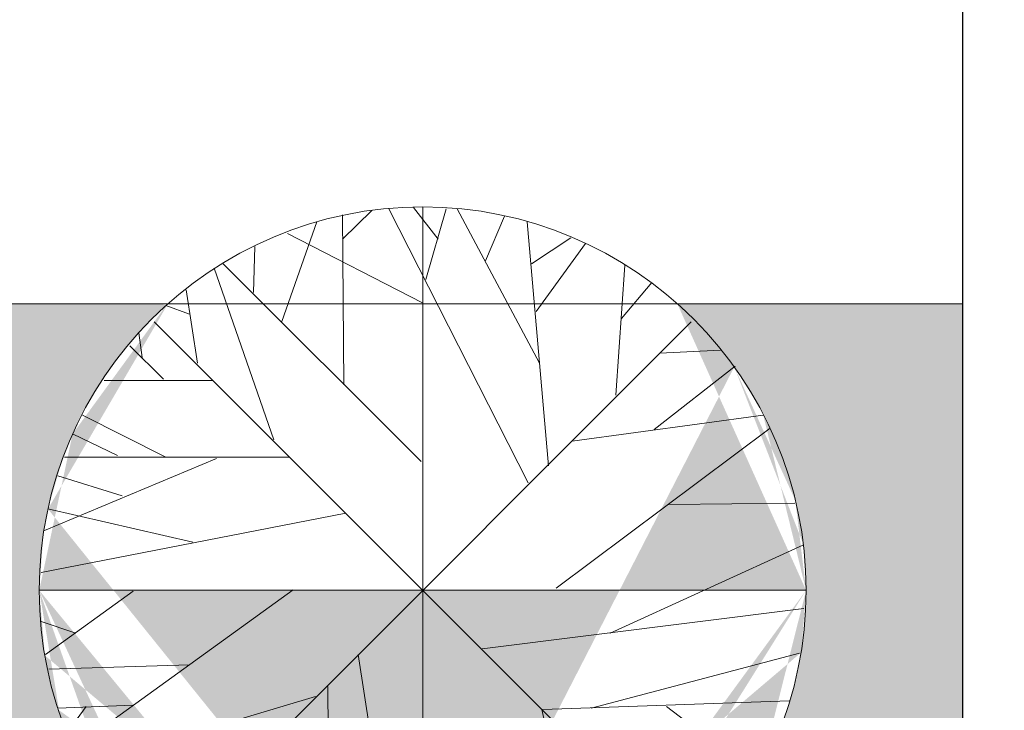
# Model space of a CAD drawing. Units: inches. Extents: x 459864 to 460310, y 324185 to 324787.
# Tile 77 of 112: x 460240 to 460271, y 324260 to 324281. Entities that reach past the tile are written whole.
import ezdxf

# ---------------------------------------------------------------- set-up
doc = ezdxf.new("R2010")
doc.units = ezdxf.units.IN
for name, color, linetype, lineweight in [('A-ANNO-DIMS', 2, 'Continuous', 18), ('C-PROP', 7, 'Continuous', 30), ('L-PLNT', 3, 'Continuous', 13), ('L-SITE-PATT', 252, 'Continuous', 13)]:
    doc.layers.add(name, color=color, linetype=linetype, lineweight=lineweight)
doc.styles.get("Standard").update_dxf_attribs({"font": 'arial.ttf'})
doc.dimstyles.new('ISO-25', dxfattribs={"dimtxt": 6, "dimasz": 2.5, "dimexe": 1.25, "dimexo": 0.625, "dimtad": 1, "dimdec": 1, "dimlunit": 3, "dimtxsty": 'Standard', "dimcen": 2.5, "dimadec": 0, "dimazin": 0, "dimtfac": 1, "dimtdec": 1, "dimtmove": 0, "dimatfit": 3, "dimfxl": 1, "dimarcsym": 0})

# ---------------------------------------------------------------- blocks, each defined once
blk = doc.blocks.new('Tree - deciduous plan')
for p, q in [((-12.5388, 54.9406), (-7.9613, 59.4546)), ((-12.3627, 32.1443), (-12.5388, 58.7776)), ((-5.3205, 59.6806), (16.5105, 16.7963)), ((2.426, 54.9406), (-1.4472, 59.9056)), ((0, 59.9996), (0, -60)), ((0.4894, 48.6208), (3.6584, 59.6806)), ((18.2711, 35.5298), (5.419, 59.6806)), ((9.8203, 51.5549), (12.8133, 58.5516)), ((-22.0458, 42.0753), (-16.5881, 57.6486)), ((19.6795, 19.5047), (16.3344, 57.6486)), ((-21.1656, 55.8436), (-0.0388, 45.0094)), ((17.0387, 51.1035), (23.2006, 55.1666)), ((17.7429, 43.6552), (25.4894, 54.2636)), ((-26.4472, 46.5894), (-26.2712, 53.8116)), ((-31.2008, 51.1035), (-0.2149, 20.1818)), ((31.6513, 50.8778), (30.2429, 30.5643)), ((-32.6092, 50.4264), (-23.2782, 23.5674)), ((31.1232, 42.5267), (35.8767, 48.1693)), ((-37.0107, 47.0408), (-35.25, 35.5298)), ((-40.1797, 44.558), (-36.4825, 43.2038)), ((42, 42), (-42, -42)), ((42, -42), (-42, 42)), ((-43.8768, 36.4326), (-44.405, 40.2696)), ((-45.8134, 38.2383), (-40.5318, 33.0471)), ((37.1091, 37.1098), (46.6161, 37.5612)), ((36.2288, 25.1474), (48.9049, 35.0784)), ((-49.8627, 32.8214), (-32.7853, 32.8214)), ((-53.2078, 27.4044), (-40.1797, 20.859)), ((23.3767, 23.3417), (53.3063, 27.4044)), ((54.3626, 25.3731), (20.9119, 0.3198)), ((-54.7923, 24.4702), (-47.75, 21.0847)), ((-32.2571, 20.6333), (-59.1937, 9.348)), ((-56.0247, 20.859), (-20.8134, 20.859)), ((-57.081, 17.9248), (-47.0458, 14.7649)), ((-58.6656, 12.7336), (-35.9543, 7.5424)), ((38.5175, 13.4107), (58.2359, 13.6364)), ((-59.7219, 2.8025), (-12.0106, 12.0565)), ((29.3626, -6.6771), (59.4682, 7.091)), ((-54.6162, -24.7335), (-20.2853, 0.0941)), ((-60, 0), (60, 0)), ((-45.2853, -0.1316), (-59.0177, -10.0627)), ((9.2922, -9.1598), (59.6443, -2.8401)), ((-59.7219, -4.8714), (-54.2641, -6.6771)), ((-10.074, -10.0627), (-2.5036, -59.7178)), ((26.3697, -18.4138), (58.9401, -9.8369)), ((-58.4895, -12.3197), (-36.4825, -11.6426)), ((-14.8275, -15.0282), (-14.6515, -57.6865)), ((-53.2078, -27.442), (-16.7641, -16.6081)), ((-57.081, -18.4138), (-45.2853, -17.9624)), ((-52.6797, -18.188), (-55.4966, -22.0251)), ((18.7992, -18.6394), (57.3556, -17.2853)), ((38.1654, -18.188), (52.426, -29.0219)), ((18.6232, -18.6394), (26.7218, -53.3981))]:
    blk.add_line(p, q)
blk.add_circle((0, 0), 60)
blk = doc.blocks.new('*D65')
at = {"layer": 'A-ANNO-DIMS', "color": 0, "lineweight": -2, "transparency": 16777216}
for p, q in [((460247.74, 324283.483), (460302.765, 324283.483)), ((460301.515, 324280.983), (460301.515, 324197.483)), ((460271.74, 324194.983), (460302.765, 324194.983))]:
    blk.add_line(p, q, dxfattribs=at)
at = {"layer": 'A-ANNO-DIMS', "color": 0, "transparency": 16777216}
for points in [[(460301.098, 324280.983), (460301.932, 324280.983), (460301.515, 324283.483)], [(460301.098, 324197.483), (460301.932, 324197.483), (460301.515, 324194.983)]]:
    blk.add_solid(points, dxfattribs=at)
at = {"layer": 'Defpoints', "color": 0, "transparency": 16777216}
for p in [(460247.115, 324283.483), (460271.115, 324194.983), (460301.515, 324194.983)]:
    blk.add_point(p, dxfattribs=at)
at = {"layer": 'A-ANNO-DIMS', "color": 0, "transparency": 16777216, "insert": (460297.788, 324239.233), "char_height": 6, "attachment_point": 5, "rotation": 90}
blk.add_mtext('7\'-4 1/2"', dxfattribs=at)

msp = doc.modelspace()

# ---------------------------------------------------------------- hatches: boundary and pattern name
at = {"layer": 'L-SITE-PATT'}
h = msp.add_hatch(dxfattribs=at)
h.set_pattern_fill('DOTS', color=256)
h.paths.add_polyline_path([(460269.804, 324283.483), (460247.115, 324283.483), (460121.929, 324283.483), (460121.929, 324252.473), (460117.429, 324252.473), (460110.124, 324252.473), (460110.124, 324243.287), (460080.83, 324243.287), (460080.83, 324252.473), (460061.115, 324252.473), (460061.115, 324251.882), (460077.909, 324251.882), (460077.909, 324199.483), (460080.83, 324199.483), (460080.83, 324207.553), (460110.124, 324207.553), (460110.124, 324199.483), (460110.813, 324199.483), (460262.115, 324199.483), (460269.804, 324199.483)], flags=17)
edge = h.paths.add_edge_path(flags=0)
edge.add_ellipse((460222.59, 324263.813), major_axis=(-8.485, 8.485), ratio=1, start_angle=405, end_angle=495, ccw=False)
edge.add_line((460214.821, 324254.66), (460214.832, 324254.666))
edge.add_ellipse((460222.59, 324263.813), major_axis=(-8.485, 8.485), ratio=1, start_angle=405, end_angle=495, ccw=False)
edge.add_line((460210.759, 324261.781), (460210.768, 324261.787))
edge.add_ellipse((460222.59, 324263.813), major_axis=(-8.485, 8.485), ratio=1, start_angle=405, end_angle=495, ccw=False)
edge.add_ellipse((460222.59, 324263.813), major_axis=(-8.485, 8.485), ratio=1, start_angle=392.754, end_angle=405, ccw=False)
edge.add_ellipse((460222.59, 324263.813), major_axis=(-8.485, 8.485), ratio=1, start_angle=380.9347, end_angle=392.754, ccw=False)
edge.add_line((460211.337, 324267.985), (460211.34, 324267.985))
edge.add_ellipse((460222.59, 324263.813), major_axis=(-8.485, 8.485), ratio=1, start_angle=380.9347, end_angle=392.754, ccw=False)
edge.add_ellipse((460222.59, 324263.813), major_axis=(-8.485, 8.485), ratio=1, start_angle=347.9015, end_angle=380.9347, ccw=False)
edge.add_ellipse((460222.59, 324263.813), major_axis=(-8.485, 8.485), ratio=1, start_angle=327.0619, end_angle=347.9015, ccw=False)
edge.add_ellipse((460222.59, 324263.813), major_axis=(-8.485, 8.485), ratio=1, start_angle=278.3246, end_angle=327.0619, ccw=False)
edge.add_line((460225.158, 324275.536), (460225.158, 324275.535))
edge.add_ellipse((460222.59, 324263.813), major_axis=(-8.485, 8.485), ratio=1, start_angle=278.3246, end_angle=327.0619, ccw=False)
edge.add_ellipse((460222.59, 324263.813), major_axis=(-8.485, 8.485), ratio=1, start_angle=260.6436, end_angle=278.3246, ccw=False)
edge.add_ellipse((460222.59, 324263.813), major_axis=(-8.485, 8.485), ratio=1, start_angle=225, end_angle=260.6436, ccw=False)
edge.add_line((460234.509, 324265.243), (460234.501, 324265.239))
edge.add_ellipse((460222.59, 324263.813), major_axis=(-8.485, 8.485), ratio=1, start_angle=225, end_angle=260.6436, ccw=False)
edge.add_ellipse((460222.59, 324263.813), major_axis=(-8.485, 8.485), ratio=1, start_angle=495, end_angle=585, ccw=False)
edge.add_line((460234.437, 324261.861), (460234.424, 324261.858))
edge.add_ellipse((460222.59, 324263.813), major_axis=(-8.485, 8.485), ratio=1, start_angle=495, end_angle=585, ccw=False)
edge.add_line((460227.95, 324253.067), (460227.946, 324253.083))
edge.add_ellipse((460222.59, 324263.813), major_axis=(-8.485, 8.485), ratio=1, start_angle=495, end_angle=585, ccw=False)
edge.add_line((460226.223, 324252.369), (460226.211, 324252.38))
edge.add_ellipse((460222.59, 324263.813), major_axis=(-8.485, 8.485), ratio=1, start_angle=495, end_angle=585, ccw=False)
h.paths.add_polyline_path([(460219.651, 324254.347), (460218.461, 324253.545), (460218.275, 324254.789), (460219.642, 324256.542), (460219.625, 324260.848), (460216.11, 324257.333), (460214.35, 324256.978), (460215.416, 324259.356), (460212.524, 324258.496), (460213.137, 324259.93), (460218.507, 324263.813), (460222.59, 324263.813), (460222.59, 324267.807), (460218.176, 324272.212), (460219.026, 324274.639), (460222.59, 324272.811), (460222.59, 324275.423), (460223.057, 324274.825), (460222.675, 324273.492), (460225.912, 324267.135), (460219.625, 324260.848)], flags=0)
edge = h.paths.add_edge_path(flags=0)
edge.add_ellipse((460194.576, 324264.046), major_axis=(-8.485, 8.485), ratio=1, start_angle=495, end_angle=585, ccw=False)
edge.add_line((460199.936, 324253.3), (460199.932, 324253.316))
edge.add_ellipse((460194.576, 324264.046), major_axis=(-8.485, 8.485), ratio=1, start_angle=495, end_angle=585, ccw=False)
edge.add_line((460198.208, 324252.603), (460198.196, 324252.613))
edge.add_ellipse((460194.576, 324264.046), major_axis=(-8.485, 8.485), ratio=1, start_angle=495, end_angle=585, ccw=False)
edge.add_ellipse((460194.576, 324264.046), major_axis=(-8.485, 8.485), ratio=1, start_angle=405, end_angle=495, ccw=False)
edge.add_line((460186.806, 324254.893), (460186.817, 324254.899))
edge.add_ellipse((460194.576, 324264.046), major_axis=(-8.485, 8.485), ratio=1, start_angle=405, end_angle=495, ccw=False)
edge.add_line((460182.744, 324262.014), (460182.753, 324262.02))
edge.add_ellipse((460194.576, 324264.046), major_axis=(-8.485, 8.485), ratio=1, start_angle=405, end_angle=495, ccw=False)
edge.add_ellipse((460194.576, 324264.046), major_axis=(-8.485, 8.485), ratio=1, start_angle=392.754, end_angle=405, ccw=False)
edge.add_ellipse((460194.576, 324264.046), major_axis=(-8.485, 8.485), ratio=1, start_angle=380.9347, end_angle=392.754, ccw=False)
edge.add_line((460183.323, 324268.218), (460183.326, 324268.218))
edge.add_ellipse((460194.576, 324264.046), major_axis=(-8.485, 8.485), ratio=1, start_angle=380.9347, end_angle=392.754, ccw=False)
edge.add_ellipse((460194.576, 324264.046), major_axis=(-8.485, 8.485), ratio=1, start_angle=347.9015, end_angle=380.9347, ccw=False)
edge.add_ellipse((460194.576, 324264.046), major_axis=(-8.485, 8.485), ratio=1, start_angle=327.0619, end_angle=347.9015, ccw=False)
edge.add_ellipse((460194.576, 324264.046), major_axis=(-8.485, 8.485), ratio=1, start_angle=278.3246, end_angle=327.0619, ccw=False)
edge.add_line((460197.144, 324275.769), (460197.143, 324275.768))
edge.add_ellipse((460194.576, 324264.046), major_axis=(-8.485, 8.485), ratio=1, start_angle=278.3246, end_angle=327.0619, ccw=False)
edge.add_ellipse((460194.576, 324264.046), major_axis=(-8.485, 8.485), ratio=1, start_angle=260.6436, end_angle=278.3246, ccw=False)
edge.add_ellipse((460194.576, 324264.046), major_axis=(-8.485, 8.485), ratio=1, start_angle=225, end_angle=260.6436, ccw=False)
edge.add_line((460206.494, 324265.476), (460206.487, 324265.473))
edge.add_ellipse((460194.576, 324264.046), major_axis=(-8.485, 8.485), ratio=1, start_angle=225, end_angle=260.6436, ccw=False)
edge.add_ellipse((460194.576, 324264.046), major_axis=(-8.485, 8.485), ratio=1, start_angle=495, end_angle=585, ccw=False)
edge.add_line((460206.422, 324262.094), (460206.409, 324262.091))
h.paths.add_polyline_path([(460191.61, 324261.081), (460191.637, 324254.58), (460190.447, 324253.778), (460190.261, 324255.023), (460191.628, 324256.775), (460191.61, 324261.081), (460188.096, 324257.566), (460186.335, 324257.211), (460187.402, 324259.589), (460184.509, 324258.729), (460185.123, 324260.163), (460190.493, 324264.046), (460194.576, 324264.046), (460194.576, 324268.04), (460190.161, 324272.446), (460191.011, 324274.872), (460194.576, 324273.044), (460194.576, 324275.657), (460195.043, 324275.058), (460194.661, 324273.725), (460197.897, 324267.368)], flags=0)
edge = h.paths.add_edge_path(flags=0)
edge.add_ellipse((460252.912, 324263.578), major_axis=(-8.485, 8.485), ratio=1, start_angle=405, end_angle=495, ccw=False)
edge.add_line((460241.081, 324261.545), (460241.089, 324261.551))
edge.add_ellipse((460252.912, 324263.578), major_axis=(-8.485, 8.485), ratio=1, start_angle=405, end_angle=495, ccw=False)
edge.add_ellipse((460252.912, 324263.578), major_axis=(-8.485, 8.485), ratio=1, start_angle=392.754, end_angle=405, ccw=False)
edge.add_ellipse((460252.912, 324263.578), major_axis=(-8.485, 8.485), ratio=1, start_angle=380.9347, end_angle=392.754, ccw=False)
edge.add_line((460241.659, 324267.749), (460241.662, 324267.749))
edge.add_ellipse((460252.912, 324263.578), major_axis=(-8.485, 8.485), ratio=1, start_angle=380.9347, end_angle=392.754, ccw=False)
edge.add_ellipse((460252.912, 324263.578), major_axis=(-8.485, 8.485), ratio=1, start_angle=347.9015, end_angle=380.9347, ccw=False)
edge.add_ellipse((460252.912, 324263.578), major_axis=(-8.485, 8.485), ratio=1, start_angle=327.0619, end_angle=347.9015, ccw=False)
edge.add_ellipse((460252.912, 324263.578), major_axis=(-8.485, 8.485), ratio=1, start_angle=278.3246, end_angle=327.0619, ccw=False)
edge.add_line((460255.48, 324275.3), (460255.479, 324275.299))
edge.add_ellipse((460252.912, 324263.578), major_axis=(-8.485, 8.485), ratio=1, start_angle=278.3246, end_angle=327.0619, ccw=False)
edge.add_ellipse((460252.912, 324263.578), major_axis=(-8.485, 8.485), ratio=1, start_angle=260.6436, end_angle=278.3246, ccw=False)
edge.add_ellipse((460252.912, 324263.578), major_axis=(-8.485, 8.485), ratio=1, start_angle=225, end_angle=260.6436, ccw=False)
edge.add_line((460264.83, 324265.007), (460264.823, 324265.004))
edge.add_ellipse((460252.912, 324263.578), major_axis=(-8.485, 8.485), ratio=1, start_angle=225, end_angle=260.6436, ccw=False)
edge.add_ellipse((460252.912, 324263.578), major_axis=(-8.485, 8.485), ratio=1, start_angle=495, end_angle=585, ccw=False)
edge.add_line((460264.758, 324261.626), (460264.745, 324261.622))
edge.add_ellipse((460252.912, 324263.578), major_axis=(-8.485, 8.485), ratio=1, start_angle=495, end_angle=585, ccw=False)
edge.add_line((460258.272, 324252.832), (460258.268, 324252.848))
edge.add_ellipse((460252.912, 324263.578), major_axis=(-8.485, 8.485), ratio=1, start_angle=495, end_angle=585, ccw=False)
edge.add_line((460256.545, 324252.134), (460256.533, 324252.144))
edge.add_ellipse((460252.912, 324263.578), major_axis=(-8.485, 8.485), ratio=1, start_angle=495, end_angle=585, ccw=False)
edge.add_ellipse((460252.912, 324263.578), major_axis=(-8.485, 8.485), ratio=1, start_angle=405, end_angle=495, ccw=False)
edge.add_line((460245.143, 324254.424), (460245.153, 324254.43))
h.paths.add_polyline_path([(460244.672, 324256.742), (460245.738, 324259.12), (460242.846, 324258.26), (460243.459, 324259.694), (460248.829, 324263.578), (460252.912, 324263.578), (460252.912, 324267.571), (460248.497, 324271.977), (460249.348, 324274.403), (460252.912, 324272.576), (460252.912, 324275.188), (460253.379, 324274.589), (460252.997, 324273.257), (460256.233, 324266.899), (460249.946, 324260.612), (460249.973, 324254.111), (460248.783, 324253.309), (460248.597, 324254.554), (460249.964, 324256.306), (460249.946, 324260.612), (460246.432, 324257.097)], flags=0)
edge = h.paths.add_edge_path(flags=0)
edge.add_ellipse((460167.439, 324262.833), major_axis=(-8.485, 8.485), ratio=1, start_angle=495, end_angle=585, ccw=False)
edge.add_line((460172.799, 324252.087), (460172.795, 324252.103))
edge.add_ellipse((460167.439, 324262.833), major_axis=(-8.485, 8.485), ratio=1, start_angle=495, end_angle=585, ccw=False)
edge.add_line((460171.071, 324251.389), (460171.059, 324251.399))
edge.add_ellipse((460167.439, 324262.833), major_axis=(-8.485, 8.485), ratio=1, start_angle=495, end_angle=585, ccw=False)
edge.add_ellipse((460167.439, 324262.833), major_axis=(-8.485, 8.485), ratio=1, start_angle=405, end_angle=495, ccw=False)
edge.add_line((460159.669, 324253.679), (460159.68, 324253.685))
edge.add_ellipse((460167.439, 324262.833), major_axis=(-8.485, 8.485), ratio=1, start_angle=405, end_angle=495, ccw=False)
edge.add_line((460155.607, 324260.8), (460155.616, 324260.806))
edge.add_ellipse((460167.439, 324262.833), major_axis=(-8.485, 8.485), ratio=1, start_angle=405, end_angle=495, ccw=False)
edge.add_ellipse((460167.439, 324262.833), major_axis=(-8.485, 8.485), ratio=1, start_angle=392.754, end_angle=405, ccw=False)
edge.add_ellipse((460167.439, 324262.833), major_axis=(-8.485, 8.485), ratio=1, start_angle=380.9347, end_angle=392.754, ccw=False)
edge.add_line((460156.185, 324267.005), (460156.189, 324267.005))
edge.add_ellipse((460167.439, 324262.833), major_axis=(-8.485, 8.485), ratio=1, start_angle=380.9347, end_angle=392.754, ccw=False)
edge.add_ellipse((460167.439, 324262.833), major_axis=(-8.485, 8.485), ratio=1, start_angle=347.9015, end_angle=380.9347, ccw=False)
edge.add_ellipse((460167.439, 324262.833), major_axis=(-8.485, 8.485), ratio=1, start_angle=327.0619, end_angle=347.9015, ccw=False)
edge.add_ellipse((460167.439, 324262.833), major_axis=(-8.485, 8.485), ratio=1, start_angle=278.3246, end_angle=327.0619, ccw=False)
edge.add_line((460170.007, 324274.556), (460170.006, 324274.554))
edge.add_ellipse((460167.439, 324262.833), major_axis=(-8.485, 8.485), ratio=1, start_angle=278.3246, end_angle=327.0619, ccw=False)
edge.add_ellipse((460167.439, 324262.833), major_axis=(-8.485, 8.485), ratio=1, start_angle=260.6436, end_angle=278.3246, ccw=False)
edge.add_ellipse((460167.439, 324262.833), major_axis=(-8.485, 8.485), ratio=1, start_angle=225, end_angle=260.6436, ccw=False)
edge.add_line((460179.357, 324264.262), (460179.35, 324264.259))
edge.add_ellipse((460167.439, 324262.833), major_axis=(-8.485, 8.485), ratio=1, start_angle=225, end_angle=260.6436, ccw=False)
edge.add_ellipse((460167.439, 324262.833), major_axis=(-8.485, 8.485), ratio=1, start_angle=495, end_angle=585, ccw=False)
edge.add_line((460179.285, 324260.881), (460179.272, 324260.877))
h.paths.add_polyline_path([(460164.473, 324259.867), (460164.5, 324253.366), (460163.31, 324252.565), (460163.124, 324253.809), (460164.491, 324255.561), (460164.473, 324259.867), (460160.958, 324256.353), (460159.198, 324255.998), (460160.265, 324258.375), (460157.372, 324257.515), (460157.986, 324258.949), (460163.356, 324262.833), (460167.439, 324262.833), (460167.439, 324266.826), (460163.024, 324271.232), (460163.874, 324273.659), (460167.439, 324271.831), (460167.439, 324274.443), (460167.905, 324273.844), (460167.524, 324272.512), (460170.76, 324266.154)], flags=0)
edge = h.paths.add_edge_path(flags=0)
edge.add_ellipse((460140.758, 324262.37), major_axis=(-8.485, 8.485), ratio=1, start_angle=495, end_angle=585, ccw=False)
edge.add_line((460146.118, 324251.624), (460146.114, 324251.639))
edge.add_ellipse((460140.758, 324262.37), major_axis=(-8.485, 8.485), ratio=1, start_angle=495, end_angle=585, ccw=False)
edge.add_line((460144.391, 324250.926), (460144.379, 324250.936))
edge.add_ellipse((460140.758, 324262.37), major_axis=(-8.485, 8.485), ratio=1, start_angle=495, end_angle=585, ccw=False)
edge.add_ellipse((460140.758, 324262.37), major_axis=(-8.485, 8.485), ratio=1, start_angle=405, end_angle=495, ccw=False)
edge.add_line((460132.989, 324253.216), (460132.999, 324253.222))
edge.add_ellipse((460140.758, 324262.37), major_axis=(-8.485, 8.485), ratio=1, start_angle=405, end_angle=495, ccw=False)
edge.add_line((460128.927, 324260.337), (460128.935, 324260.343))
edge.add_ellipse((460140.758, 324262.37), major_axis=(-8.485, 8.485), ratio=1, start_angle=405, end_angle=495, ccw=False)
edge.add_ellipse((460140.758, 324262.37), major_axis=(-8.485, 8.485), ratio=1, start_angle=392.754, end_angle=405, ccw=False)
edge.add_ellipse((460140.758, 324262.37), major_axis=(-8.485, 8.485), ratio=1, start_angle=380.9347, end_angle=392.754, ccw=False)
edge.add_line((460129.505, 324266.541), (460129.508, 324266.541))
edge.add_ellipse((460140.758, 324262.37), major_axis=(-8.485, 8.485), ratio=1, start_angle=380.9347, end_angle=392.754, ccw=False)
edge.add_ellipse((460140.758, 324262.37), major_axis=(-8.485, 8.485), ratio=1, start_angle=347.9015, end_angle=380.9347, ccw=False)
edge.add_ellipse((460140.758, 324262.37), major_axis=(-8.485, 8.485), ratio=1, start_angle=327.0619, end_angle=347.9015, ccw=False)
edge.add_ellipse((460140.758, 324262.37), major_axis=(-8.485, 8.485), ratio=1, start_angle=278.3246, end_angle=327.0619, ccw=False)
edge.add_line((460143.326, 324274.092), (460143.325, 324274.091))
edge.add_ellipse((460140.758, 324262.37), major_axis=(-8.485, 8.485), ratio=1, start_angle=278.3246, end_angle=327.0619, ccw=False)
edge.add_ellipse((460140.758, 324262.37), major_axis=(-8.485, 8.485), ratio=1, start_angle=260.6436, end_angle=278.3246, ccw=False)
edge.add_ellipse((460140.758, 324262.37), major_axis=(-8.485, 8.485), ratio=1, start_angle=225, end_angle=260.6436, ccw=False)
edge.add_line((460152.677, 324263.799), (460152.669, 324263.796))
edge.add_ellipse((460140.758, 324262.37), major_axis=(-8.485, 8.485), ratio=1, start_angle=225, end_angle=260.6436, ccw=False)
edge.add_ellipse((460140.758, 324262.37), major_axis=(-8.485, 8.485), ratio=1, start_angle=495, end_angle=585, ccw=False)
edge.add_line((460152.604, 324260.418), (460152.592, 324260.414))
h.paths.add_polyline_path([(460137.792, 324259.404), (460137.819, 324252.903), (460136.629, 324252.101), (460136.443, 324253.346), (460137.81, 324255.098), (460137.792, 324259.404), (460134.278, 324255.889), (460132.518, 324255.534), (460133.584, 324257.912), (460130.692, 324257.052), (460131.305, 324258.486), (460136.675, 324262.37), (460140.758, 324262.37), (460140.758, 324266.363), (460136.343, 324270.769), (460137.194, 324273.195), (460140.758, 324271.367), (460140.758, 324273.98), (460141.225, 324273.381), (460140.843, 324272.049), (460144.079, 324265.691)], flags=0)
h.paths.add_polyline_path([(460110.124, 324227.414), (460080.83, 324227.414), (460080.83, 324235.484), (460110.124, 324235.484)], flags=16)
h.paths.add_polyline_path([(460110.124, 324220.797), (460110.124, 324212.727), (460080.83, 324212.727), (460080.83, 324220.797)], flags=16)
h.paths.add_polyline_path([(460269.804, 324283.483), (460247.115, 324283.483), (460121.929, 324283.483), (460121.929, 324252.473), (460117.429, 324252.473), (460110.124, 324252.473), (460110.124, 324243.287), (460080.83, 324243.287), (460080.83, 324252.473), (460061.115, 324252.473), (460061.115, 324251.882), (460077.909, 324251.882), (460077.909, 324199.483), (460080.83, 324199.483), (460080.83, 324207.553), (460110.124, 324207.553), (460110.124, 324199.483), (460262.115, 324199.483), (460269.804, 324199.483)], flags=17)
h.paths.add_polyline_path([(460219.651, 324254.347), (460218.461, 324253.545), (460218.275, 324254.789), (460219.642, 324256.542), (460219.625, 324260.848), (460216.11, 324257.333), (460214.35, 324256.978), (460215.416, 324259.356), (460212.524, 324258.496), (460213.137, 324259.93), (460218.507, 324263.813), (460222.59, 324263.813), (460220.18, 324266.223), (460215.461, 324265.308), (460211.835, 324266.137), (460216.247, 324267.985), (460218.418, 324267.985), (460222.59, 324263.813), (460222.59, 324267.807), (460218.176, 324272.212), (460219.026, 324274.639), (460222.59, 324272.811), (460222.59, 324275.423), (460223.057, 324274.825), (460222.675, 324273.492), (460225.912, 324267.135), (460222.59, 324263.813), (460231.383, 324263.813), (460228.485, 324262.488), (460224.425, 324261.978), (460228.68, 324257.724), (460228.966, 324254.791), (460227.142, 324256.537), (460227.542, 324254.819), (460227.333, 324253.614), (460222.59, 324259.985), (460222.59, 324255.497), (460221.377, 324256.541), (460220.576, 324261.799), (460219.625, 324260.848)], flags=0)
h.paths.add_polyline_path([(460199.127, 324256.77), (460199.528, 324255.052), (460199.319, 324253.848), (460194.576, 324260.218), (460194.576, 324255.73), (460193.363, 324256.774), (460192.561, 324262.032), (460191.61, 324261.081), (460191.637, 324254.58), (460190.447, 324253.778), (460190.261, 324255.023), (460191.628, 324256.775), (460191.61, 324261.081), (460188.096, 324257.566), (460186.335, 324257.211), (460187.402, 324259.589), (460184.509, 324258.729), (460185.123, 324260.163), (460190.493, 324264.046), (460194.576, 324264.046), (460192.166, 324266.456), (460187.446, 324265.541), (460183.82, 324266.37), (460188.232, 324268.218), (460190.404, 324268.218), (460194.576, 324264.046), (460194.576, 324268.04), (460190.161, 324272.446), (460191.011, 324274.872), (460194.576, 324273.044), (460194.576, 324275.657), (460195.043, 324275.058), (460194.661, 324273.725), (460197.897, 324267.368), (460194.576, 324264.046), (460203.368, 324264.046), (460200.47, 324262.721), (460196.411, 324262.212), (460200.665, 324257.957), (460200.951, 324255.024)], flags=0)
h.paths.add_polyline_path([(460244.672, 324256.742), (460245.738, 324259.12), (460242.846, 324258.26), (460243.459, 324259.694), (460248.829, 324263.578), (460252.912, 324263.578), (460250.502, 324265.987), (460245.783, 324265.072), (460242.156, 324265.901), (460246.568, 324267.749), (460248.74, 324267.749), (460252.912, 324263.578), (460252.912, 324267.571), (460248.497, 324271.977), (460249.348, 324274.403), (460252.912, 324272.576), (460252.912, 324275.188), (460253.379, 324274.589), (460252.997, 324273.257), (460256.233, 324266.899), (460252.912, 324263.578), (460261.705, 324263.578), (460258.806, 324262.252), (460254.747, 324261.743), (460259.002, 324257.488), (460259.288, 324254.555), (460257.463, 324256.301), (460257.864, 324254.583), (460257.655, 324253.379), (460252.912, 324259.749), (460252.912, 324255.261), (460251.699, 324256.305), (460250.897, 324261.563), (460249.946, 324260.612), (460249.973, 324254.111), (460248.783, 324253.309), (460248.597, 324254.554), (460249.964, 324256.306), (460249.946, 324260.612), (460246.432, 324257.097)], flags=0)
h.paths.add_polyline_path([(460173.528, 324256.743), (460173.814, 324253.811), (460171.99, 324255.556), (460172.39, 324253.838), (460172.182, 324252.634), (460167.439, 324259.004), (460167.439, 324254.516), (460166.226, 324255.56), (460165.424, 324260.818), (460164.473, 324259.867), (460164.5, 324253.366), (460163.31, 324252.565), (460163.124, 324253.809), (460164.491, 324255.561), (460164.473, 324259.867), (460160.958, 324256.353), (460159.198, 324255.998), (460160.265, 324258.375), (460157.372, 324257.515), (460157.986, 324258.949), (460163.356, 324262.833), (460167.439, 324262.833), (460165.029, 324265.243), (460160.309, 324264.327), (460156.683, 324265.156), (460161.095, 324267.005), (460163.267, 324267.005), (460167.439, 324262.833), (460167.439, 324266.826), (460163.024, 324271.232), (460163.874, 324273.659), (460167.439, 324271.831), (460167.439, 324274.443), (460167.905, 324273.844), (460167.524, 324272.512), (460170.76, 324266.154), (460167.439, 324262.833), (460176.231, 324262.833), (460173.333, 324261.507), (460169.274, 324260.998)], flags=0)
h.paths.add_polyline_path([(460146.848, 324256.28), (460147.134, 324253.347), (460145.31, 324255.093), (460145.71, 324253.375), (460145.501, 324252.171), (460140.758, 324258.541), (460140.758, 324254.053), (460139.545, 324255.097), (460138.744, 324260.355), (460137.792, 324259.404), (460137.819, 324252.903), (460136.629, 324252.101), (460136.443, 324253.346), (460137.81, 324255.098), (460137.792, 324259.404), (460134.278, 324255.889), (460132.518, 324255.534), (460133.584, 324257.912), (460130.692, 324257.052), (460131.305, 324258.486), (460136.675, 324262.37), (460140.758, 324262.37), (460138.348, 324264.779), (460133.629, 324263.864), (460130.002, 324264.693), (460134.414, 324266.541), (460136.586, 324266.541), (460140.758, 324262.37), (460140.758, 324266.363), (460136.343, 324270.769), (460137.194, 324273.195), (460140.758, 324271.367), (460140.758, 324273.98), (460141.225, 324273.381), (460140.843, 324272.049), (460144.079, 324265.691), (460140.758, 324262.37), (460149.551, 324262.37), (460146.653, 324261.044), (460142.593, 324260.535)], flags=0)
edge = h.paths.add_edge_path()
edge.add_line((460269.804, 324272.549), (460260.881, 324272.549))
edge.add_ellipse((460252.912, 324263.578), major_axis=(-8.485, 8.485), ratio=1, start_angle=260.6436, end_angle=273.3846, ccw=False)
edge.add_line((460262.283, 324271.092), (460262.261, 324271.091))
edge.add_ellipse((460252.912, 324263.578), major_axis=(-8.485, 8.485), ratio=1, start_angle=260.6436, end_angle=273.3846, ccw=False)
edge.add_ellipse((460252.912, 324263.578), major_axis=(-8.485, 8.485), ratio=1, start_angle=225, end_angle=260.6436, ccw=False)
edge.add_line((460263.609, 324269.063), (460263.572, 324269.058))
edge.add_ellipse((460252.912, 324263.578), major_axis=(-8.485, 8.485), ratio=1, start_angle=225, end_angle=260.6436, ccw=False)
edge.add_line((460264.615, 324266.306), (460264.585, 324266.305))
edge.add_ellipse((460252.912, 324263.578), major_axis=(-8.485, 8.485), ratio=1, start_angle=225, end_angle=260.6436, ccw=False)
edge.add_line((460264.83, 324265.007), (460264.823, 324265.004))
edge.add_ellipse((460252.912, 324263.578), major_axis=(-8.485, 8.485), ratio=1, start_angle=225, end_angle=260.6436, ccw=False)
edge.add_ellipse((460252.912, 324263.578), major_axis=(-8.485, 8.485), ratio=1, start_angle=495, end_angle=585, ccw=False)
edge.add_line((460264.758, 324261.626), (460264.745, 324261.622))
edge.add_ellipse((460252.912, 324263.578), major_axis=(-8.485, 8.485), ratio=1, start_angle=495, end_angle=585, ccw=False)
edge.add_line((460263.442, 324257.739), (460263.389, 324257.779))
edge.add_ellipse((460252.912, 324263.578), major_axis=(-8.485, 8.485), ratio=1, start_angle=495, end_angle=585, ccw=False)
edge.add_line((460258.128, 324252.744), (460258.102, 324252.779))
edge.add_ellipse((460252.912, 324263.578), major_axis=(-8.485, 8.485), ratio=1, start_angle=495, end_angle=585, ccw=False)
edge.add_line((460256.545, 324252.134), (460256.533, 324252.144))
edge.add_ellipse((460252.912, 324263.578), major_axis=(-8.485, 8.485), ratio=1, start_angle=495, end_angle=585, ccw=False)
edge.add_ellipse((460252.912, 324263.578), major_axis=(-8.485, 8.485), ratio=1, start_angle=405, end_angle=495, ccw=False)
edge.add_line((460250.594, 324251.78), (460250.605, 324251.82))
edge.add_ellipse((460252.912, 324263.578), major_axis=(-8.485, 8.485), ratio=1, start_angle=405, end_angle=495, ccw=False)
edge.add_line((460245.143, 324254.424), (460245.153, 324254.43))
edge.add_ellipse((460252.912, 324263.578), major_axis=(-8.485, 8.485), ratio=1, start_angle=405, end_angle=495, ccw=False)
edge.add_line((460243.525, 324256.059), (460243.56, 324256.091))
edge.add_ellipse((460252.912, 324263.578), major_axis=(-8.485, 8.485), ratio=1, start_angle=405, end_angle=495, ccw=False)
edge.add_line((460241.44, 324259.893), (460241.522, 324259.896))
edge.add_ellipse((460252.912, 324263.578), major_axis=(-8.485, 8.485), ratio=1, start_angle=405, end_angle=495, ccw=False)
edge.add_line((460241.081, 324261.545), (460241.089, 324261.551))
edge.add_ellipse((460252.912, 324263.578), major_axis=(-8.485, 8.485), ratio=1, start_angle=405, end_angle=495, ccw=False)
edge.add_ellipse((460252.912, 324263.578), major_axis=(-8.485, 8.485), ratio=1, start_angle=392.754, end_angle=405, ccw=False)
edge.add_line((460241.05, 324265.438), (460241.063, 324265.443))
edge.add_ellipse((460252.912, 324263.578), major_axis=(-8.485, 8.485), ratio=1, start_angle=392.754, end_angle=405, ccw=False)
edge.add_ellipse((460252.912, 324263.578), major_axis=(-8.485, 8.485), ratio=1, start_angle=380.9347, end_angle=392.754, ccw=False)
edge.add_line((460241.452, 324267.176), (460241.469, 324267.171))
edge.add_ellipse((460252.912, 324263.578), major_axis=(-8.485, 8.485), ratio=1, start_angle=380.9347, end_angle=392.754, ccw=False)
edge.add_line((460241.659, 324267.749), (460241.662, 324267.749))
edge.add_ellipse((460252.912, 324263.578), major_axis=(-8.485, 8.485), ratio=1, start_angle=380.9347, end_angle=392.754, ccw=False)
edge.add_ellipse((460252.912, 324263.578), major_axis=(-8.485, 8.485), ratio=1, start_angle=356.6154, end_angle=380.9347, ccw=False)
edge.add_line((460244.88, 324272.488), (460244.713, 324272.549))
edge.add_line((460244.713, 324272.549), (460230.817, 324272.549))
edge.add_ellipse((460222.59, 324263.813), major_axis=(-8.485, 8.485), ratio=1, start_angle=260.6436, end_angle=271.7178, ccw=False)
edge.add_ellipse((460222.59, 324263.813), major_axis=(-8.485, 8.485), ratio=1, start_angle=225, end_angle=260.6436, ccw=False)
edge.add_line((460233.287, 324269.299), (460233.25, 324269.294))
edge.add_ellipse((460222.59, 324263.813), major_axis=(-8.485, 8.485), ratio=1, start_angle=225, end_angle=260.6436, ccw=False)
edge.add_line((460234.294, 324266.541), (460234.264, 324266.541))
edge.add_ellipse((460222.59, 324263.813), major_axis=(-8.485, 8.485), ratio=1, start_angle=225, end_angle=260.6436, ccw=False)
edge.add_line((460234.509, 324265.243), (460234.501, 324265.239))
edge.add_ellipse((460222.59, 324263.813), major_axis=(-8.485, 8.485), ratio=1, start_angle=225, end_angle=260.6436, ccw=False)
edge.add_ellipse((460222.59, 324263.813), major_axis=(-8.485, 8.485), ratio=1, start_angle=495, end_angle=585, ccw=False)
edge.add_line((460234.437, 324261.861), (460234.424, 324261.858))
edge.add_ellipse((460222.59, 324263.813), major_axis=(-8.485, 8.485), ratio=1, start_angle=495, end_angle=585, ccw=False)
edge.add_line((460233.121, 324257.975), (460233.068, 324258.015))
edge.add_ellipse((460222.59, 324263.813), major_axis=(-8.485, 8.485), ratio=1, start_angle=495, end_angle=585, ccw=False)
edge.add_line((460227.806, 324252.979), (460227.78, 324253.014))
edge.add_ellipse((460222.59, 324263.813), major_axis=(-8.485, 8.485), ratio=1, start_angle=495, end_angle=585, ccw=False)
edge.add_line((460226.223, 324252.369), (460226.211, 324252.38))
edge.add_ellipse((460222.59, 324263.813), major_axis=(-8.485, 8.485), ratio=1, start_angle=495, end_angle=585, ccw=False)
edge.add_ellipse((460222.59, 324263.813), major_axis=(-8.485, 8.485), ratio=1, start_angle=405, end_angle=495, ccw=False)
edge.add_line((460220.272, 324252.016), (460220.283, 324252.055))
edge.add_ellipse((460222.59, 324263.813), major_axis=(-8.485, 8.485), ratio=1, start_angle=405, end_angle=495, ccw=False)
edge.add_line((460214.821, 324254.66), (460214.832, 324254.666))
edge.add_ellipse((460222.59, 324263.813), major_axis=(-8.485, 8.485), ratio=1, start_angle=405, end_angle=495, ccw=False)
edge.add_line((460213.203, 324256.295), (460213.239, 324256.327))
edge.add_ellipse((460222.59, 324263.813), major_axis=(-8.485, 8.485), ratio=1, start_angle=405, end_angle=495, ccw=False)
edge.add_line((460211.118, 324260.128), (460211.201, 324260.131))
edge.add_ellipse((460222.59, 324263.813), major_axis=(-8.485, 8.485), ratio=1, start_angle=405, end_angle=495, ccw=False)
edge.add_line((460210.759, 324261.781), (460210.768, 324261.787))
edge.add_ellipse((460222.59, 324263.813), major_axis=(-8.485, 8.485), ratio=1, start_angle=405, end_angle=495, ccw=False)
edge.add_ellipse((460222.59, 324263.813), major_axis=(-8.485, 8.485), ratio=1, start_angle=392.754, end_angle=405, ccw=False)
edge.add_line((460210.729, 324265.673), (460210.741, 324265.678))
edge.add_ellipse((460222.59, 324263.813), major_axis=(-8.485, 8.485), ratio=1, start_angle=392.754, end_angle=405, ccw=False)
edge.add_ellipse((460222.59, 324263.813), major_axis=(-8.485, 8.485), ratio=1, start_angle=380.9347, end_angle=392.754, ccw=False)
edge.add_line((460211.13, 324267.412), (460211.147, 324267.407))
edge.add_ellipse((460222.59, 324263.813), major_axis=(-8.485, 8.485), ratio=1, start_angle=380.9347, end_angle=392.754, ccw=False)
edge.add_line((460211.337, 324267.985), (460211.34, 324267.985))
edge.add_ellipse((460222.59, 324263.813), major_axis=(-8.485, 8.485), ratio=1, start_angle=380.9347, end_angle=392.754, ccw=False)
edge.add_ellipse((460222.59, 324263.813), major_axis=(-8.485, 8.485), ratio=1, start_angle=358.2822, end_angle=380.9347, ccw=False)
edge.add_line((460213.705, 324271.902), (460213.709, 324271.869))
edge.add_ellipse((460222.59, 324263.813), major_axis=(-8.485, 8.485), ratio=1, start_angle=358.2822, end_angle=380.9347, ccw=False)
edge.add_line((460214.363, 324272.549), (460203.078, 324272.549))
edge.add_line((460203.078, 324272.549), (460203.06, 324272.531))
edge.add_ellipse((460194.576, 324264.046), major_axis=(-8.485, 8.485), ratio=1, start_angle=260.6436, end_angle=270.1168, ccw=False)
edge.add_line((460203.957, 324271.561), (460203.921, 324271.56))
edge.add_ellipse((460194.576, 324264.046), major_axis=(-8.485, 8.485), ratio=1, start_angle=260.6436, end_angle=270.1168, ccw=False)
edge.add_ellipse((460194.576, 324264.046), major_axis=(-8.485, 8.485), ratio=1, start_angle=225, end_angle=260.6436, ccw=False)
edge.add_line((460205.272, 324269.532), (460205.235, 324269.527))
edge.add_ellipse((460194.576, 324264.046), major_axis=(-8.485, 8.485), ratio=1, start_angle=225, end_angle=260.6436, ccw=False)
edge.add_line((460206.279, 324266.774), (460206.249, 324266.774))
edge.add_ellipse((460194.576, 324264.046), major_axis=(-8.485, 8.485), ratio=1, start_angle=225, end_angle=260.6436, ccw=False)
edge.add_line((460206.494, 324265.476), (460206.487, 324265.473))
edge.add_ellipse((460194.576, 324264.046), major_axis=(-8.485, 8.485), ratio=1, start_angle=225, end_angle=260.6436, ccw=False)
edge.add_ellipse((460194.576, 324264.046), major_axis=(-8.485, 8.485), ratio=1, start_angle=495, end_angle=585, ccw=False)
edge.add_line((460206.422, 324262.094), (460206.409, 324262.091))
edge.add_ellipse((460194.576, 324264.046), major_axis=(-8.485, 8.485), ratio=1, start_angle=495, end_angle=585, ccw=False)
edge.add_line((460205.106, 324258.208), (460205.053, 324258.248))
edge.add_ellipse((460194.576, 324264.046), major_axis=(-8.485, 8.485), ratio=1, start_angle=495, end_angle=585, ccw=False)
edge.add_line((460199.792, 324253.212), (460199.766, 324253.248))
edge.add_ellipse((460194.576, 324264.046), major_axis=(-8.485, 8.485), ratio=1, start_angle=495, end_angle=585, ccw=False)
edge.add_line((460198.208, 324252.603), (460198.196, 324252.613))
edge.add_ellipse((460194.576, 324264.046), major_axis=(-8.485, 8.485), ratio=1, start_angle=495, end_angle=585, ccw=False)
edge.add_ellipse((460194.576, 324264.046), major_axis=(-8.485, 8.485), ratio=1, start_angle=405, end_angle=495, ccw=False)
edge.add_line((460192.258, 324252.249), (460192.268, 324252.289))
edge.add_ellipse((460194.576, 324264.046), major_axis=(-8.485, 8.485), ratio=1, start_angle=405, end_angle=495, ccw=False)
edge.add_line((460186.806, 324254.893), (460186.817, 324254.899))
edge.add_ellipse((460194.576, 324264.046), major_axis=(-8.485, 8.485), ratio=1, start_angle=405, end_angle=495, ccw=False)
edge.add_line((460185.188, 324256.528), (460185.224, 324256.56))
edge.add_ellipse((460194.576, 324264.046), major_axis=(-8.485, 8.485), ratio=1, start_angle=405, end_angle=495, ccw=False)
edge.add_line((460183.104, 324260.362), (460183.186, 324260.365))
edge.add_ellipse((460194.576, 324264.046), major_axis=(-8.485, 8.485), ratio=1, start_angle=405, end_angle=495, ccw=False)
edge.add_line((460182.744, 324262.014), (460182.753, 324262.02))
edge.add_ellipse((460194.576, 324264.046), major_axis=(-8.485, 8.485), ratio=1, start_angle=405, end_angle=495, ccw=False)
edge.add_ellipse((460194.576, 324264.046), major_axis=(-8.485, 8.485), ratio=1, start_angle=392.754, end_angle=405, ccw=False)
edge.add_line((460182.714, 324265.906), (460182.726, 324265.912))
edge.add_ellipse((460194.576, 324264.046), major_axis=(-8.485, 8.485), ratio=1, start_angle=392.754, end_angle=405, ccw=False)
edge.add_ellipse((460194.576, 324264.046), major_axis=(-8.485, 8.485), ratio=1, start_angle=380.9347, end_angle=392.754, ccw=False)
edge.add_line((460183.116, 324267.645), (460183.133, 324267.64))
edge.add_ellipse((460194.576, 324264.046), major_axis=(-8.485, 8.485), ratio=1, start_angle=380.9347, end_angle=392.754, ccw=False)
edge.add_line((460183.323, 324268.218), (460183.326, 324268.218))
edge.add_ellipse((460194.576, 324264.046), major_axis=(-8.485, 8.485), ratio=1, start_angle=380.9347, end_angle=392.754, ccw=False)
edge.add_ellipse((460194.576, 324264.046), major_axis=(-8.485, 8.485), ratio=1, start_angle=359.8832, end_angle=380.9347, ccw=False)
edge.add_line((460184.491, 324270.611), (460184.553, 324270.611))
edge.add_ellipse((460194.576, 324264.046), major_axis=(-8.485, 8.485), ratio=1, start_angle=359.8832, end_angle=380.9347, ccw=False)
edge.add_line((460185.346, 324271.76), (460185.379, 324271.728))
edge.add_ellipse((460194.576, 324264.046), major_axis=(-8.485, 8.485), ratio=1, start_angle=359.8832, end_angle=380.9347, ccw=False)
edge.add_line((460185.697, 324272.086), (460185.633, 324272.549))
edge.add_line((460185.633, 324272.549), (460174.683, 324272.549))
edge.add_line((460174.683, 324272.549), (460174.606, 324272.457))
edge.add_ellipse((460167.439, 324262.833), major_axis=(-8.485, 8.485), ratio=1, start_angle=260.6436, end_angle=278.3246, ccw=False)
edge.add_ellipse((460167.439, 324262.833), major_axis=(-8.485, 8.485), ratio=1, start_angle=225, end_angle=260.6436, ccw=False)
edge.add_line((460178.135, 324268.318), (460178.098, 324268.313))
edge.add_ellipse((460167.439, 324262.833), major_axis=(-8.485, 8.485), ratio=1, start_angle=225, end_angle=260.6436, ccw=False)
edge.add_line((460179.142, 324265.561), (460179.112, 324265.56))
edge.add_ellipse((460167.439, 324262.833), major_axis=(-8.485, 8.485), ratio=1, start_angle=225, end_angle=260.6436, ccw=False)
edge.add_line((460179.357, 324264.262), (460179.35, 324264.259))
edge.add_ellipse((460167.439, 324262.833), major_axis=(-8.485, 8.485), ratio=1, start_angle=225, end_angle=260.6436, ccw=False)
edge.add_ellipse((460167.439, 324262.833), major_axis=(-8.485, 8.485), ratio=1, start_angle=495, end_angle=585, ccw=False)
edge.add_line((460179.285, 324260.881), (460179.272, 324260.877))
edge.add_ellipse((460167.439, 324262.833), major_axis=(-8.485, 8.485), ratio=1, start_angle=495, end_angle=585, ccw=False)
edge.add_line((460177.969, 324256.994), (460177.916, 324257.034))
edge.add_ellipse((460167.439, 324262.833), major_axis=(-8.485, 8.485), ratio=1, start_angle=495, end_angle=585, ccw=False)
edge.add_line((460172.655, 324251.999), (460172.629, 324252.034))
edge.add_ellipse((460167.439, 324262.833), major_axis=(-8.485, 8.485), ratio=1, start_angle=495, end_angle=585, ccw=False)
edge.add_line((460171.071, 324251.389), (460171.059, 324251.399))
edge.add_ellipse((460167.439, 324262.833), major_axis=(-8.485, 8.485), ratio=1, start_angle=495, end_angle=585, ccw=False)
edge.add_ellipse((460167.439, 324262.833), major_axis=(-8.485, 8.485), ratio=1, start_angle=405, end_angle=495, ccw=False)
edge.add_line((460165.121, 324251.036), (460165.131, 324251.075))
edge.add_ellipse((460167.439, 324262.833), major_axis=(-8.485, 8.485), ratio=1, start_angle=405, end_angle=495, ccw=False)
edge.add_line((460159.669, 324253.679), (460159.68, 324253.685))
edge.add_ellipse((460167.439, 324262.833), major_axis=(-8.485, 8.485), ratio=1, start_angle=405, end_angle=495, ccw=False)
edge.add_line((460158.051, 324255.314), (460158.087, 324255.347))
edge.add_ellipse((460167.439, 324262.833), major_axis=(-8.485, 8.485), ratio=1, start_angle=405, end_angle=495, ccw=False)
edge.add_line((460155.967, 324259.148), (460156.049, 324259.151))
edge.add_ellipse((460167.439, 324262.833), major_axis=(-8.485, 8.485), ratio=1, start_angle=405, end_angle=495, ccw=False)
edge.add_line((460155.607, 324260.8), (460155.616, 324260.806))
edge.add_ellipse((460167.439, 324262.833), major_axis=(-8.485, 8.485), ratio=1, start_angle=405, end_angle=495, ccw=False)
edge.add_ellipse((460167.439, 324262.833), major_axis=(-8.485, 8.485), ratio=1, start_angle=392.754, end_angle=405, ccw=False)
edge.add_line((460155.577, 324264.693), (460155.589, 324264.698))
edge.add_ellipse((460167.439, 324262.833), major_axis=(-8.485, 8.485), ratio=1, start_angle=392.754, end_angle=405, ccw=False)
edge.add_ellipse((460167.439, 324262.833), major_axis=(-8.485, 8.485), ratio=1, start_angle=380.9347, end_angle=392.754, ccw=False)
edge.add_line((460155.979, 324266.432), (460155.996, 324266.426))
edge.add_ellipse((460167.439, 324262.833), major_axis=(-8.485, 8.485), ratio=1, start_angle=380.9347, end_angle=392.754, ccw=False)
edge.add_line((460156.185, 324267.005), (460156.189, 324267.005))
edge.add_ellipse((460167.439, 324262.833), major_axis=(-8.485, 8.485), ratio=1, start_angle=380.9347, end_angle=392.754, ccw=False)
edge.add_ellipse((460167.439, 324262.833), major_axis=(-8.485, 8.485), ratio=1, start_angle=350.9345, end_angle=380.9347, ccw=False)
edge.add_line((460157.363, 324269.397), (460157.414, 324269.397))
edge.add_ellipse((460167.439, 324262.833), major_axis=(-8.485, 8.485), ratio=1, start_angle=350.9345, end_angle=380.9347, ccw=False)
edge.add_line((460158.221, 324270.535), (460158.236, 324270.519))
edge.add_ellipse((460167.439, 324262.833), major_axis=(-8.485, 8.485), ratio=1, start_angle=350.9345, end_angle=380.9347, ccw=False)
edge.add_line((460159.379, 324271.753), (460159.419, 324271.738))
edge.add_ellipse((460167.439, 324262.833), major_axis=(-8.485, 8.485), ratio=1, start_angle=350.9345, end_angle=380.9347, ccw=False)
edge.add_line((460160.396, 324272.549), (460147.112, 324272.549))
edge.add_ellipse((460140.758, 324262.37), major_axis=(-8.485, 8.485), ratio=1, start_angle=278.3246, end_angle=283.0261, ccw=False)
edge.add_ellipse((460140.758, 324262.37), major_axis=(-8.485, 8.485), ratio=1, start_angle=260.6436, end_angle=278.3246, ccw=False)
edge.add_ellipse((460140.758, 324262.37), major_axis=(-8.485, 8.485), ratio=1, start_angle=225, end_angle=260.6436, ccw=False)
edge.add_line((460151.455, 324267.855), (460151.418, 324267.85))
edge.add_ellipse((460140.758, 324262.37), major_axis=(-8.485, 8.485), ratio=1, start_angle=225, end_angle=260.6436, ccw=False)
edge.add_line((460152.462, 324265.098), (460152.431, 324265.097))
edge.add_ellipse((460140.758, 324262.37), major_axis=(-8.485, 8.485), ratio=1, start_angle=225, end_angle=260.6436, ccw=False)
edge.add_line((460152.677, 324263.799), (460152.669, 324263.796))
edge.add_ellipse((460140.758, 324262.37), major_axis=(-8.485, 8.485), ratio=1, start_angle=225, end_angle=260.6436, ccw=False)
edge.add_ellipse((460140.758, 324262.37), major_axis=(-8.485, 8.485), ratio=1, start_angle=495, end_angle=585, ccw=False)
edge.add_line((460152.604, 324260.418), (460152.592, 324260.414))
edge.add_ellipse((460140.758, 324262.37), major_axis=(-8.485, 8.485), ratio=1, start_angle=495, end_angle=585, ccw=False)
edge.add_line((460151.288, 324256.531), (460151.235, 324256.571))
edge.add_ellipse((460140.758, 324262.37), major_axis=(-8.485, 8.485), ratio=1, start_angle=495, end_angle=585, ccw=False)
edge.add_line((460145.974, 324251.535), (460145.948, 324251.571))
edge.add_ellipse((460140.758, 324262.37), major_axis=(-8.485, 8.485), ratio=1, start_angle=495, end_angle=585, ccw=False)
edge.add_line((460144.391, 324250.926), (460144.379, 324250.936))
edge.add_ellipse((460140.758, 324262.37), major_axis=(-8.485, 8.485), ratio=1, start_angle=495, end_angle=585, ccw=False)
edge.add_ellipse((460140.758, 324262.37), major_axis=(-8.485, 8.485), ratio=1, start_angle=405, end_angle=495, ccw=False)
edge.add_line((460138.44, 324250.572), (460138.451, 324250.612))
edge.add_ellipse((460140.758, 324262.37), major_axis=(-8.485, 8.485), ratio=1, start_angle=405, end_angle=495, ccw=False)
edge.add_line((460132.989, 324253.216), (460132.999, 324253.222))
edge.add_ellipse((460140.758, 324262.37), major_axis=(-8.485, 8.485), ratio=1, start_angle=405, end_angle=495, ccw=False)
edge.add_line((460131.371, 324254.851), (460131.406, 324254.883))
edge.add_ellipse((460140.758, 324262.37), major_axis=(-8.485, 8.485), ratio=1, start_angle=405, end_angle=495, ccw=False)
edge.add_line((460129.286, 324258.685), (460129.369, 324258.688))
edge.add_ellipse((460140.758, 324262.37), major_axis=(-8.485, 8.485), ratio=1, start_angle=405, end_angle=495, ccw=False)
edge.add_line((460128.927, 324260.337), (460128.935, 324260.343))
edge.add_ellipse((460140.758, 324262.37), major_axis=(-8.485, 8.485), ratio=1, start_angle=405, end_angle=495, ccw=False)
edge.add_ellipse((460140.758, 324262.37), major_axis=(-8.485, 8.485), ratio=1, start_angle=392.754, end_angle=405, ccw=False)
edge.add_line((460128.896, 324264.23), (460128.909, 324264.235))
edge.add_ellipse((460140.758, 324262.37), major_axis=(-8.485, 8.485), ratio=1, start_angle=392.754, end_angle=405, ccw=False)
edge.add_ellipse((460140.758, 324262.37), major_axis=(-8.485, 8.485), ratio=1, start_angle=380.9347, end_angle=392.754, ccw=False)
edge.add_line((460129.298, 324265.968), (460129.315, 324265.963))
edge.add_ellipse((460140.758, 324262.37), major_axis=(-8.485, 8.485), ratio=1, start_angle=380.9347, end_angle=392.754, ccw=False)
edge.add_line((460129.505, 324266.541), (460129.508, 324266.541))
edge.add_ellipse((460140.758, 324262.37), major_axis=(-8.485, 8.485), ratio=1, start_angle=380.9347, end_angle=392.754, ccw=False)
edge.add_ellipse((460140.758, 324262.37), major_axis=(-8.485, 8.485), ratio=1, start_angle=347.9015, end_angle=380.9347, ccw=False)
edge.add_line((460130.697, 324268.934), (460130.727, 324268.934))
edge.add_ellipse((460140.758, 324262.37), major_axis=(-8.485, 8.485), ratio=1, start_angle=347.9015, end_angle=380.9347, ccw=False)
edge.add_line((460131.869, 324270.48), (460131.879, 324270.413))
edge.add_ellipse((460140.758, 324262.37), major_axis=(-8.485, 8.485), ratio=1, start_angle=347.9015, end_angle=380.9347, ccw=False)
edge.add_line((460132.734, 324271.277), (460132.705, 324271.287))
edge.add_ellipse((460140.758, 324262.37), major_axis=(-8.485, 8.485), ratio=1, start_angle=347.9015, end_angle=380.9347, ccw=False)
edge.add_line((460134.24, 324272.445), (460134.204, 324272.549))
edge.add_line((460134.204, 324272.549), (460121.929, 324272.549))
edge.add_line((460121.929, 324272.549), (460121.929, 324252.473))
edge.add_line((460121.929, 324252.473), (460117.429, 324252.473))
edge.add_line((460117.429, 324252.473), (460110.124, 324252.473))
edge.add_line((460110.124, 324252.473), (460110.124, 324243.287))
edge.add_line((460110.124, 324243.287), (460080.83, 324243.287))
edge.add_line((460080.83, 324243.287), (460080.83, 324252.473))
edge.add_line((460080.83, 324252.473), (460061.115, 324252.473))
edge.add_line((460061.115, 324252.473), (460061.115, 324251.882))
edge.add_line((460061.115, 324251.882), (460077.909, 324251.882))
edge.add_line((460077.909, 324251.882), (460077.909, 324199.483))
edge.add_line((460077.909, 324199.483), (460080.83, 324199.483))
edge.add_line((460080.83, 324199.483), (460080.83, 324207.553))
edge.add_line((460080.83, 324207.553), (460110.124, 324207.553))
edge.add_line((460110.124, 324207.553), (460110.124, 324199.483))
edge.add_line((460110.124, 324199.483), (460110.813, 324199.483))
edge.add_line((460110.813, 324199.483), (460262.115, 324199.483))
edge.add_line((460262.115, 324199.483), (460269.804, 324199.483))
edge.add_line((460269.804, 324199.483), (460269.804, 324272.549))

# ---------------------------------------------------------------- linework, layer by layer
at = {"layer": 'C-PROP'}
msp.add_line((460269.804, 324466.483), (460269.804, 324199.483), dxfattribs=at)
at = {"layer": 'L-PLNT'}
msp.add_line((460121.929, 324272.549), (460269.804, 324272.549), dxfattribs=at)

# ---------------------------------------------------------------- block references
at = {"layer": 'L-PLNT', "xscale": 0.2, "yscale": 0.2}
msp.add_blockref('Tree - deciduous plan', (460252.912, 324263.578), dxfattribs=at)

# ---------------------------------------------------------------- dimensions: what is measured, and where the dimension line sits
at = {"layer": 'A-ANNO-DIMS'}
dim = msp.add_linear_dim(base=(460301.515, 324194.983), p1=(460247.115, 324283.483), p2=(460271.115, 324194.983), angle=90, dimstyle='ISO-25', override={"dimdec": 1, "dimlfac": 1, "dimrnd": 0, "dimzin": 1, "dimdsep": 46, "dimlunit": 4, "dimfrac": 2}, dxfattribs=at)
dim.commit()
dim.dimension.update_dxf_attribs({"geometry": '*D65', "text_midpoint": (460297.788, 324239.233)})

doc.saveas('drawing.dxf')
